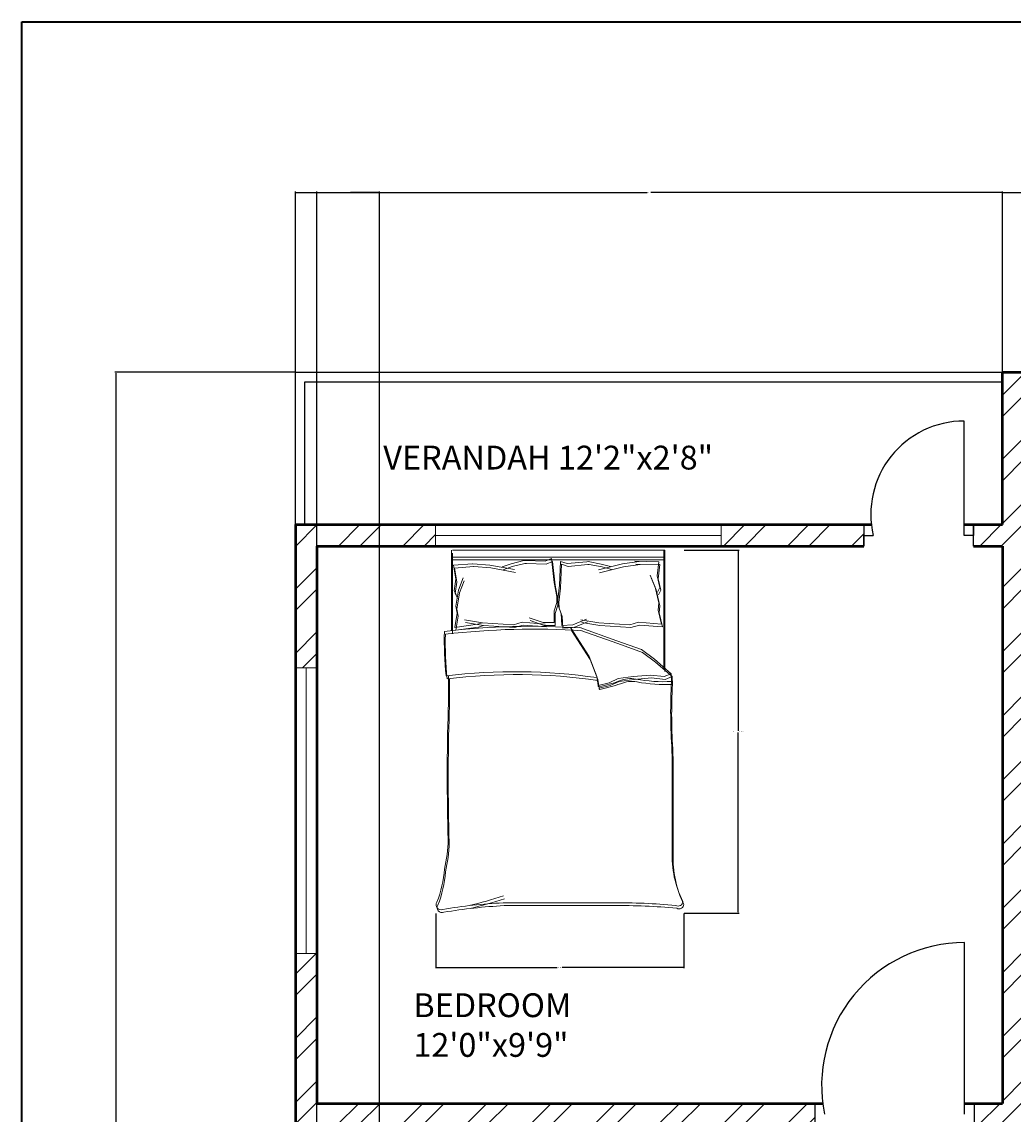
# Model space of a CAD drawing. Units: inches. Extents: x 2129 to 2642, y 1542 to 2414.
# Tile 6 of 9: x 2129 to 2338, y 2184 to 2414. Entities that reach past the tile are written whole.
import ezdxf

# ---------------------------------------------------------------- set-up
doc = ezdxf.new("R2010")
doc.units = ezdxf.units.IN
for name, color, linetype, lineweight in [('A-ANNO-DIMS', 2, 'Continuous', 18), ('A-ANNO-TTLB', 7, 'Continuous', 35), ('A-AREA-IDEN', 7, 'Continuous', 18), ('A-DOOR', 3, 'Continuous', 25), ('A-FLOR-RAIL', 80, 'Continuous', 25), ('A-FURN', 8, 'Continuous', 18), ('A-GLAZ', 4, 'Continuous', 18), ('A-WALL', 7, 'Continuous', 50), ('A-WALL-PATT', 252, 'Continuous', 13)]:
    doc.layers.add(name, color=color, linetype=linetype, lineweight=lineweight)
doc.styles.get("Standard").update_dxf_attribs({"font": 'arial.ttf'})
doc.dimstyles.get("Standard").update_dxf_attribs({"dimtxt": 0.18, "dimasz": 0.18, "dimexe": 0.18, "dimexo": 0.0625, "dimgap": 0.09, "dimtad": 0, "dimtih": 1, "dimtoh": 1, "dimdec": 4, "dimzin": 0, "dimdsep": 46, "dimtxsty": 'Standard', "dimcen": 0.09, "dimadec": 0, "dimazin": 0, "dimtfac": 1, "dimtdec": 4, "dimtofl": 0, "dimtmove": 0, "dimatfit": 3, "dimfxl": 1, "dimtolj": 1, "dimtzin": 0, "dimarcsym": 0})

# ---------------------------------------------------------------- blocks, each defined once
blk = doc.blocks.new('BED-DOUBLE')
for p, q in [((3.24, 59.14), (3.24, 76.05)), ((3.25, 59.14), (3.25, 76.05)), ((48.08, 76.05), (3.46, 76.05)), ((47.87, 76.05), (47.87, 51.2)), ((47.87, 76.05), (47.87, 51.2)), ((48.08, 76.05), (48.08, 75.45)), ((3.24, 74.61), (47.87, 74.61)), ((3.25, 74.61), (47.87, 74.61)), ((3.46, 58.54), (3.46, 75.45)), ((3.46, 58.54), (3.46, 75.45)), ((3.46, 74.02), (48.08, 74.02)), ((3.46, 74.02), (48.08, 74.02)), ((15.76, 73.22), (18.46, 73.9)), ((15.76, 73.22), (18.46, 73.9)), ((18.46, 73.9), (18.76, 73.9)), ((18.46, 73.9), (18.76, 73.9)), ((18.76, 73.9), (22.91, 73.76)), ((18.76, 73.9), (22.91, 73.76)), ((22.91, 73.76), (24.26, 74.3)), ((22.91, 73.76), (24.26, 74.3)), ((23.12, 73.16), (24.47, 73.7)), ((23.12, 73.16), (24.47, 73.7)), ((24.26, 74.3), (24.8, 69.31)), ((24.26, 74.3), (24.8, 69.31)), ((24.47, 73.7), (25.01, 68.71)), ((24.47, 73.7), (25.01, 68.71)), ((26.12, 73.72), (25.9, 68.7)), ((26.12, 73.72), (25.9, 68.7)), ((27.5, 73.27), (26.12, 73.72)), ((27.5, 73.27), (26.12, 73.72)), ((31.64, 73.66), (27.5, 73.27)), ((31.64, 73.66), (27.5, 73.27)), ((31.94, 73.68), (31.64, 73.66)), ((31.94, 73.68), (31.64, 73.66)), ((34.68, 73.17), (31.94, 73.68)), ((34.67, 73.17), (31.94, 73.68)), ((42.68, 73.67), (39.14, 73.18)), ((42.68, 73.67), (39.14, 73.18)), ((46.79, 73.66), (41.75, 73.75)), ((41.75, 73.75), (42.68, 73.67)), ((46.79, 73.66), (41.75, 73.75)), ((41.75, 73.75), (42.68, 73.67)), ((46.79, 73.66), (46.44, 70.66)), ((46.79, 73.66), (46.44, 70.66)), ((48.08, 75.45), (48.08, 50.6)), ((48.08, 75.45), (48.08, 50.6)), ((3.64, 72.93), (7.64, 73.24)), ((3.64, 72.93), (7.64, 73.24)), ((3.64, 72.95), (4.18, 69.98)), ((3.64, 72.95), (4.18, 69.98)), ((3.85, 72.33), (7.85, 72.64)), ((3.85, 72.33), (7.85, 72.64)), ((3.85, 72.35), (4.39, 69.38)), ((3.85, 72.35), (4.39, 69.38)), ((7.64, 73.24), (7.74, 73.22)), ((7.64, 73.24), (7.74, 73.22)), ((7.74, 73.22), (11.31, 72.95)), ((7.74, 73.22), (11.31, 72.95)), ((7.85, 72.64), (7.95, 72.62)), ((7.85, 72.64), (7.95, 72.62)), ((7.95, 72.62), (11.52, 72.35)), ((7.95, 72.62), (11.52, 72.35)), ((11.31, 72.95), (16.44, 72.01)), ((11.31, 72.95), (16.44, 72.01)), ((11.52, 72.35), (16.65, 71.41)), ((11.52, 72.35), (16.65, 71.41)), ((13.87, 72.55), (15.76, 73.22)), ((13.87, 72.55), (15.76, 73.22)), ((14.08, 71.95), (15.97, 72.62)), ((14.08, 71.95), (15.97, 72.62)), ((15.97, 72.62), (18.67, 73.3)), ((15.97, 72.62), (18.67, 73.3)), ((18.67, 73.3), (18.97, 73.3)), ((18.67, 73.3), (18.97, 73.3)), ((18.97, 73.3), (23.12, 73.16)), ((18.97, 73.3), (23.12, 73.16)), ((26.34, 73.12), (26.11, 68.1)), ((26.34, 73.12), (26.11, 68.1)), ((27.72, 72.67), (26.34, 73.12)), ((27.72, 72.67), (26.34, 73.12)), ((31.85, 73.06), (27.72, 72.67)), ((31.85, 73.06), (27.72, 72.67)), ((32.15, 73.08), (31.85, 73.06)), ((32.15, 73.08), (31.85, 73.06)), ((34.89, 72.58), (32.15, 73.08)), ((34.89, 72.58), (32.15, 73.08)), ((39.14, 73.18), (34.08, 71.92)), ((39.14, 73.18), (34.08, 71.92)), ((39.35, 72.58), (34.29, 71.32)), ((39.35, 72.58), (34.29, 71.32)), ((36.6, 72.62), (34.67, 73.17)), ((36.6, 72.62), (34.68, 73.17)), ((36.82, 72.02), (34.89, 72.58)), ((36.82, 72.02), (34.89, 72.58)), ((42.9, 73.08), (39.35, 72.58)), ((42.9, 73.08), (39.35, 72.58)), ((47.01, 73.06), (41.96, 73.15)), ((41.96, 73.15), (42.9, 73.08)), ((47.01, 73.06), (41.96, 73.15)), ((41.96, 73.15), (42.9, 73.08)), ((47.01, 73.06), (46.65, 70.06)), ((47.01, 73.06), (46.65, 70.06)), ((4.18, 69.98), (3.77, 67.55)), ((4.18, 69.98), (3.77, 67.55)), ((4.39, 69.38), (3.98, 66.95)), ((4.39, 69.38), (3.99, 66.95)), ((4.72, 67.69), (5.66, 70.25)), ((4.72, 67.69), (5.66, 70.25)), ((4.93, 67.09), (5.87, 69.65)), ((4.93, 67.09), (5.87, 69.65)), ((24.8, 69.31), (25.34, 66.34)), ((24.8, 69.31), (25.34, 66.34)), ((46.04, 68.34), (44.94, 70.84)), ((46.04, 68.34), (44.94, 70.84)), ((46.26, 67.74), (45.15, 70.24)), ((46.26, 67.74), (45.15, 70.24)), ((46.44, 70.66), (46.99, 68.26)), ((46.44, 70.66), (46.99, 68.26)), ((46.65, 70.06), (47.21, 67.66)), ((46.65, 70.06), (47.21, 67.66)), ((3.77, 67.55), (4.31, 66.61)), ((3.77, 67.55), (4.31, 66.61)), ((3.98, 66.95), (4.52, 66.01)), ((3.99, 66.95), (4.53, 66.01)), ((4.18, 64.31), (4.72, 67.69)), ((4.18, 64.31), (4.72, 67.69)), ((4.39, 63.71), (4.93, 67.09)), ((4.39, 63.71), (4.93, 67.09)), ((25.01, 68.71), (25.55, 65.74)), ((25.01, 68.71), (25.55, 65.74)), ((25.9, 68.7), (25.54, 65.7)), ((25.9, 68.7), (25.54, 65.7)), ((26.11, 68.1), (25.76, 65.11)), ((26.11, 68.1), (25.76, 65.11)), ((46.79, 65), (46.04, 68.34)), ((46.79, 65), (46.04, 68.34)), ((47.01, 64.41), (46.26, 67.74)), ((47.01, 64.41), (46.26, 67.74)), ((46.99, 68.26), (46.51, 67.28)), ((46.99, 68.26), (46.51, 67.28)), ((47.21, 67.66), (46.73, 66.69)), ((47.21, 67.66), (46.73, 66.69)), ((4.45, 62.82), (4.18, 64.31)), ((4.45, 62.82), (4.18, 64.31)), ((25.34, 65.12), (24.8, 63.36)), ((25.34, 65.12), (24.8, 63.36)), ((25.55, 64.52), (25.01, 62.77)), ((25.55, 64.52), (25.01, 62.77)), ((25.34, 66.34), (25.34, 65.12)), ((25.34, 66.34), (25.34, 65.12)), ((25.54, 65.7), (25.62, 64.49)), ((25.54, 65.7), (25.62, 64.49)), ((25.55, 65.74), (25.55, 64.52)), ((25.55, 65.74), (25.55, 64.52)), ((25.62, 64.49), (26.27, 62.77)), ((25.62, 64.49), (26.27, 62.77)), ((25.76, 65.11), (25.83, 63.89)), ((25.76, 65.11), (25.83, 63.89)), ((46.62, 63.5), (46.79, 65)), ((46.62, 63.5), (46.79, 65)), ((46.83, 62.91), (47.01, 64.41)), ((46.83, 62.91), (47.01, 64.41)), ((3.91, 59.85), (4.45, 62.82)), ((3.91, 59.85), (4.45, 62.82)), ((4.12, 59.26), (4.66, 62.23)), ((4.12, 59.26), (4.66, 62.23)), ((4.66, 62.23), (4.39, 63.71)), ((4.66, 62.23), (4.39, 63.71)), ((24.8, 63.36), (24.8, 60.86)), ((24.8, 63.36), (24.8, 60.86)), ((25.01, 62.77), (25.01, 60.26)), ((25.01, 62.77), (25.01, 60.26)), ((25.83, 63.89), (26.48, 62.18)), ((25.83, 63.89), (26.48, 62.18)), ((26.27, 62.77), (26.42, 60.27)), ((26.27, 62.77), (26.42, 60.27)), ((26.48, 62.18), (26.64, 59.68)), ((26.48, 62.18), (26.64, 59.68)), ((47.34, 60.57), (46.62, 63.5)), ((47.34, 60.57), (46.62, 63.5)), ((47.55, 59.98), (46.83, 62.91)), ((47.55, 59.98), (46.83, 62.91)), ((8.67, 60.53), (3.91, 59.85)), ((8.67, 60.53), (3.91, 59.85)), ((8.88, 59.93), (4.12, 59.26)), ((8.88, 59.93), (4.12, 59.26)), ((5.96, 61.45), (9.72, 60.83)), ((5.96, 61.45), (9.72, 60.83)), ((6.17, 60.86), (9.94, 60.23)), ((6.17, 60.86), (9.94, 60.23)), ((9.72, 60.83), (8.67, 60.53)), ((9.72, 60.83), (8.67, 60.53)), ((9.94, 60.23), (8.88, 59.93)), ((9.94, 60.23), (8.88, 59.93)), ((9.72, 60.83), (16.27, 60.43)), ((9.72, 60.83), (16.27, 60.43)), ((9.94, 60.23), (16.48, 59.83)), ((9.94, 60.23), (16.48, 59.83)), ((16.27, 60.43), (18.1, 60.95)), ((16.27, 60.43), (18.1, 60.95)), ((16.48, 59.83), (18.31, 60.35)), ((16.48, 59.83), (18.31, 60.35)), ((18.1, 60.95), (22.89, 60.57)), ((18.1, 60.95), (22.89, 60.57)), ((18.31, 60.35), (23.11, 59.98)), ((18.31, 60.35), (23.1, 59.98)), ((22.51, 60.86), (19.57, 61.88)), ((22.51, 60.86), (19.57, 61.88)), ((22.72, 60.26), (19.78, 61.28)), ((22.72, 60.26), (19.78, 61.28)), ((24.8, 60.86), (22.51, 60.86)), ((24.8, 60.86), (22.51, 60.86)), ((25.01, 60.26), (22.72, 60.26)), ((25.01, 60.26), (22.72, 60.26)), ((26.42, 60.27), (28.71, 60.42)), ((26.42, 60.27), (28.71, 60.42)), ((26.64, 59.68), (28.93, 59.82)), ((26.64, 59.68), (28.93, 59.82)), ((28.25, 59.82), (32.17, 53.75)), ((28.25, 59.82), (32.17, 53.75)), ((28.71, 60.42), (31.58, 61.62)), ((28.71, 60.42), (31.58, 61.62)), ((28.93, 59.82), (31.79, 61.02)), ((28.93, 59.82), (31.79, 61.02)), ((37.95, 57.08), (30.17, 59.82)), ((37.95, 57.08), (30.17, 59.82)), ((30.41, 61.45), (34.17, 60.83)), ((30.41, 61.45), (34.17, 60.83)), ((30.62, 60.86), (34.39, 60.23)), ((30.62, 60.86), (34.38, 60.23)), ((34.17, 60.83), (40.72, 60.43)), ((34.17, 60.83), (40.72, 60.43)), ((34.38, 60.23), (40.93, 59.83)), ((34.39, 60.23), (40.93, 59.83)), ((40.72, 60.43), (42.55, 60.95)), ((40.72, 60.43), (42.55, 60.95)), ((40.93, 59.83), (42.76, 60.35)), ((40.93, 59.83), (42.76, 60.35)), ((42.55, 60.95), (47.34, 60.57)), ((42.55, 60.95), (47.34, 60.57)), ((42.76, 60.35), (47.55, 59.98)), ((42.76, 60.35), (47.55, 59.98)), ((28.47, 59.22), (32.38, 53.16)), ((28.47, 59.22), (32.38, 53.16)), ((38.16, 56.48), (30.38, 59.22)), ((38.16, 56.48), (30.38, 59.22)), ((43.16, 55.2), (37.95, 57.08)), ((43.16, 55.2), (37.95, 57.08)), ((43.37, 54.6), (38.16, 56.48)), ((43.37, 54.6), (38.16, 56.48)), ((45.91, 53.17), (43.16, 55.2)), ((45.91, 53.17), (43.16, 55.2)), ((32.17, 53.75), (33.76, 49.56)), ((32.17, 53.75), (33.76, 49.56)), ((32.38, 53.16), (33.97, 48.96)), ((32.38, 53.16), (33.97, 48.96)), ((46.12, 52.58), (43.37, 54.6)), ((46.12, 52.58), (43.37, 54.6)), ((49.37, 50.14), (45.91, 53.17)), ((49.36, 50.14), (45.91, 53.17)), ((49.58, 49.54), (46.12, 52.58)), ((49.58, 49.54), (46.12, 52.58)), ((33.76, 49.56), (34.05, 47.68)), ((33.76, 49.56), (34.05, 47.68)), ((33.97, 48.96), (34.26, 47.09)), ((33.97, 48.96), (34.26, 47.09)), ((34.05, 47.68), (36.36, 48.26)), ((34.05, 47.68), (36.36, 48.26)), ((36.36, 48.26), (38.24, 49.13)), ((36.36, 48.26), (38.24, 49.13)), ((36.57, 47.66), (38.45, 48.53)), ((36.57, 47.66), (38.45, 48.53)), ((38.24, 49.13), (41.42, 49.56)), ((38.24, 49.13), (41.42, 49.56)), ((38.45, 48.53), (41.64, 48.96)), ((38.45, 48.53), (41.64, 48.96)), ((41.42, 49.56), (45.04, 49.85)), ((41.42, 49.56), (45.04, 49.85)), ((41.64, 48.96), (45.25, 49.25)), ((41.64, 48.96), (45.25, 49.25)), ((45.04, 49.85), (47.93, 49.56)), ((45.04, 49.85), (47.93, 49.56)), ((45.25, 49.25), (48.14, 48.96)), ((45.25, 49.25), (48.14, 48.96)), ((47.93, 49.56), (49.37, 50.14)), ((47.93, 49.56), (49.36, 50.14)), ((48.14, 48.96), (49.58, 49.54)), ((48.14, 48.96), (49.58, 49.54)), ((49.44, 48.51), (49.36, 50.14, 3.61)), ((49.44, 48.51), (49.37, 50.14, 3.61)), ((49.65, 47.91), (49.58, 49.54, 3.61)), ((49.65, 47.91), (49.58, 49.54, 3.61)), ((34.26, 47.09), (36.57, 47.66)), ((34.26, 47.09), (36.57, 47.66)), ((14.07, 2.05), (37.05, 2.05)), ((14.07, 2.05), (37.05, 2.05)), ((14.28, 1.46), (37.26, 1.46)), ((14.28, 1.46), (37.26, 1.46))]:
    blk.add_line(p, q)
for centre, radius, start, end in [((19.94, -93.94), 154.04, 86.0865, 96.7821), ((19.94, -93.94), 154.04, 86.0865, 96.7821), ((79.52, 57.28), 77.79, 178.7218, 185.604), ((79.52, 57.28), 77.79, 178.7218, 185.604), ((79.73, 56.69), 77.79, 178.7218, 185.604), ((79.73, 56.69), 77.79, 178.7218, 185.604), ((20.16, -94.54), 154.04, 86.0865, 96.7821), ((20.16, -94.54), 154.04, 86.0865, 96.7821), ((16.58, -69.91), 120.47, 81.7845, 96.9006), ((16.58, -69.91), 120.47, 81.7845, 96.9006), ((16.79, -70.51), 120.47, 81.7845, 96.9006), ((16.79, -70.51), 120.47, 81.7845, 96.9006), ((-156.22, 46.94), 158.84, 358.4762, 1.0082), ((-156.22, 46.94), 158.84, 358.4762, 1.0082), ((-156.01, 46.34), 158.84, 358.4762, 1.0082), ((-156.01, 46.34), 158.84, 358.4762, 1.0082), ((29.09, 74.66), 27.69, 280.6617, 289.8806), ((29.09, 74.66), 27.69, 280.6617, 289.8806), ((40.85, 43.3), 5.81, 78.6608, 113.7384), ((40.85, 43.3), 5.81, 78.6608, 113.7384), ((41.06, 42.71), 5.81, 78.6608, 113.7384), ((41.06, 42.71), 5.81, 78.6608, 113.7384), ((47.93, 82.26), 33.79, 259.8763, 272.5657), ((47.93, 82.26), 33.79, 259.8763, 272.5657), ((48.14, 81.67), 33.79, 259.8763, 272.5657), ((48.14, 81.67), 33.79, 259.8763, 272.5657), ((170.19, 42.14), 120.92, 176.9791, 183.8365), ((170.19, 42.14), 120.92, 176.9791, 183.8365), ((34.21, 47.62), 0.172, 160.2464, 271.1377), ((34.21, 47.62), 0.172, 160.2464, 271.1377), ((34.42, 47.03), 0.172, 160.2464, 271.1377), ((34.42, 47.03), 0.172, 160.2464, 271.1377), ((29.3, 74.07), 27.69, 280.6617, 289.8806), ((29.3, 74.07), 27.69, 280.6617, 289.8806), ((170.4, 41.54), 120.92, 176.9791, 183.8365), ((170.4, 41.54), 120.92, 176.9791, 183.8365), ((452.7, 28.79), 450.36, 178.2277, 181.7185), ((452.7, 28.79), 450.36, 178.2277, 181.7185), ((452.91, 28.19), 450.36, 178.2277, 181.7185), ((452.91, 28.19), 450.36, 178.2277, 181.7185), ((-4210.02, 12.72), 4259.62, 0.00217, 0.28689), ((-4210.02, 12.72), 4259.62, 0.00217, 0.28689), ((-4209.81, 12.12), 4259.62, 0.00217, 0.28689), ((-4209.81, 12.12), 4259.62, 0.00217, 0.28689), ((-25.12, 15.81), 27.67, 346.0648, 358.9113), ((-25.12, 15.81), 27.67, 346.0648, 358.9113), ((-24.9, 15.21), 27.67, 346.0648, 358.9113), ((-24.9, 15.21), 27.67, 346.0648, 358.9113), ((71.11, 11.93), 21.54, 177.4714, 206.4681), ((71.11, 11.93), 21.54, 177.4714, 206.4681), ((71.33, 11.33), 21.54, 177.4714, 206.4681), ((71.32, 11.33), 21.54, 177.4714, 206.4681), ((-20.22, 10.43), 22, 337.9751, 356.652), ((-20.22, 10.43), 22, 337.9751, 356.652), ((-20.01, 9.83), 22, 337.9751, 356.652), ((-20.01, 9.83), 22, 337.9751, 356.652), ((-16.08, 98.19), 99.41, 283.3832, 287.7053), ((-16.08, 98.19), 99.41, 283.3832, 287.7053), ((-15.87, 97.59), 99.41, 283.3832, 287.7053), ((-15.87, 97.59), 99.41, 283.3832, 287.7053), ((50.81, 2.4), 1.03, 242.6588, 356.02), ((50.81, 2.4), 1.03, 242.6588, 356.02), ((1.02, 1.61), 1.02, 146.1736, 293.4781), ((1.02, 1.61), 1.02, 146.1736, 293.4781), ((1.23, 1.01), 1.02, 146.1736, 293.4781), ((1.23, 1.01), 1.02, 146.1736, 293.4781), ((20.01, -111.48), 113.69, 92.9958, 99.4091), ((20.01, -111.48), 113.69, 92.9958, 99.4091), ((20.22, -112.08), 113.69, 92.9958, 99.4091), ((20.22, -112.08), 113.69, 92.9958, 99.4091), ((38.43, -122.17), 124.23, 84.4998, 90.6351), ((38.43, -122.17), 124.23, 84.4998, 90.6351), ((38.64, -122.76), 124.23, 84.4998, 90.6351), ((38.64, -122.76), 124.23, 84.4998, 90.6351), ((51.02, 1.81), 1.03, 242.6588, 356.02), ((51.02, 1.81), 1.03, 242.6588, 356.02)]:
    blk.add_arc(centre, radius, start, end)
blk = doc.blocks.new('WIN-60-A')
for p, q in [((0, 4.5), (0, 0)), ((60, 2.25), (60, 4.5)), ((60, 4.5), (60, 0)), ((0, 0), (0, 2.25)), ((0, 2.25), (60, 2.25))]:
    blk.add_line(p, q)
blk = doc.blocks.new('*D12')
at = {"layer": 'A-ANNO-DIMS', "color": 0, "lineweight": -2, "transparency": 16777216}
for p, q in [((2268.55, 2302.83), (2280.09, 2302.83)), ((2279.91, 2302.65), (2279.91, 2264.94)), ((2279.91, 2226.87), (2279.91, 2264.58)), ((2268.55, 2226.69), (2280.09, 2226.69))]:
    blk.add_line(p, q, dxfattribs=at)
at = {"layer": 'A-ANNO-DIMS', "color": 0, "transparency": 16777216}
for points in [[(2279.88, 2302.65), (2279.94, 2302.65), (2279.91, 2302.83)], [(2279.88, 2226.87), (2279.94, 2226.87), (2279.91, 2226.69)]]:
    blk.add_solid(points, dxfattribs=at)
at = {"layer": 'Defpoints', "color": 0, "transparency": 16777216}
for p in [(2268.49, 2302.83), (2279.91, 2302.83), (2268.49, 2226.69)]:
    blk.add_point(p, dxfattribs=at)
at = {"layer": 'A-ANNO-DIMS', "color": 0, "transparency": 16777216, "insert": (2279.91, 2264.76), "char_height": 0.18, "attachment_point": 5}
blk.add_mtext('\\A1;DOUBLE BED 76 TYP.', dxfattribs=at)
blk = doc.blocks.new('*D13')
at = {"layer": 'A-ANNO-DIMS', "color": 0, "lineweight": -2, "transparency": 16777216}
for p, q in [((2216.36, 2226.62), (2216.36, 2215.09)), ((2268.49, 2226.62), (2268.49, 2215.09)), ((2216.54, 2215.27), (2241.9, 2215.27)), ((2268.31, 2215.27), (2242.96, 2215.27))]:
    blk.add_line(p, q, dxfattribs=at)
at = {"layer": 'A-ANNO-DIMS', "color": 0, "transparency": 16777216}
for points in [[(2216.54, 2215.3), (2216.54, 2215.24), (2216.36, 2215.27)], [(2268.31, 2215.3), (2268.31, 2215.24), (2268.49, 2215.27)]]:
    blk.add_solid(points, dxfattribs=at)
at = {"layer": 'Defpoints', "color": 0, "transparency": 16777216}
for p in [(2216.36, 2226.69), (2268.49, 2226.69), (2268.49, 2215.27)]:
    blk.add_point(p, dxfattribs=at)
at = {"layer": 'A-ANNO-DIMS', "color": 0, "transparency": 16777216, "insert": (2242.43, 2215.27), "char_height": 0.18, "attachment_point": 5}
blk.add_mtext('\\A1;52 TYP.', dxfattribs=at)
blk = doc.blocks.new('*D35')
at = {"layer": 'A-ANNO-DIMS', "color": 0, "lineweight": -2, "transparency": 16777216}
for p, q in [((2186.84, 2340.22), (2148.97, 2340.22)), ((2149.15, 2340.04), (2149.15, 2003.15)), ((2149.15, 1665.9), (2149.15, 2002.79)), ((2186.84, 1665.72), (2148.97, 1665.72))]:
    blk.add_line(p, q, dxfattribs=at)
at = {"layer": 'A-ANNO-DIMS', "color": 0, "transparency": 16777216}
for points in [[(2149.12, 2340.04), (2149.18, 2340.04), (2149.15, 2340.22)], [(2149.12, 1665.9), (2149.18, 1665.9), (2149.15, 1665.72)]]:
    blk.add_solid(points, dxfattribs=at)
at = {"layer": 'Defpoints', "color": 0, "transparency": 16777216}
for p in [(2149.15, 2340.22), (2186.9, 2340.22), (2186.9, 1665.72)]:
    blk.add_point(p, dxfattribs=at)
at = {"layer": 'A-ANNO-DIMS', "color": 0, "transparency": 16777216, "insert": (2149.15, 2002.97), "char_height": 0.18, "attachment_point": 5}
blk.add_mtext('\\A1;674.5', dxfattribs=at)
blk = doc.blocks.new('*D36')
at = {"layer": 'A-ANNO-DIMS', "color": 0, "lineweight": -2, "transparency": 16777216}
for p, q in [((2186.9, 2340.28), (2186.9, 2378.15)), ((2187.08, 2377.97), (2260.77, 2377.97)), ((2335.22, 2377.97), (2261.54, 2377.97)), ((2335.4, 2340.28), (2335.4, 2378.15))]:
    blk.add_line(p, q, dxfattribs=at)
at = {"layer": 'A-ANNO-DIMS', "color": 0, "transparency": 16777216}
for points in [[(2187.08, 2378), (2187.08, 2377.94), (2186.9, 2377.97)], [(2335.22, 2378), (2335.22, 2377.94), (2335.4, 2377.97)]]:
    blk.add_solid(points, dxfattribs=at)
at = {"layer": 'Defpoints', "color": 0, "transparency": 16777216}
for p in [(2335.4, 2377.97), (2186.9, 2340.22), (2335.4, 2340.22)]:
    blk.add_point(p, dxfattribs=at)
at = {"layer": 'A-ANNO-DIMS', "color": 0, "transparency": 16777216, "insert": (2261.15, 2377.97), "char_height": 0.18, "attachment_point": 5}
blk.add_mtext('\\A1;148.5', dxfattribs=at)
blk = doc.blocks.new('*D37')
at = {"layer": 'A-ANNO-DIMS', "color": 0, "lineweight": -2, "transparency": 16777216}
for p, q in [((2335.4, 2340.28), (2335.4, 2378.15)), ((2335.58, 2377.97), (2387.62, 2377.97)), ((2440.22, 2377.97), (2388.19, 2377.97)), ((2440.4, 2340.28), (2440.4, 2378.15))]:
    blk.add_line(p, q, dxfattribs=at)
at = {"layer": 'A-ANNO-DIMS', "color": 0, "transparency": 16777216}
for points in [[(2335.58, 2378), (2335.58, 2377.94), (2335.4, 2377.97)], [(2440.22, 2378), (2440.22, 2377.94), (2440.4, 2377.97)]]:
    blk.add_solid(points, dxfattribs=at)
at = {"layer": 'Defpoints', "color": 0, "transparency": 16777216}
for p in [(2440.4, 2377.97), (2335.4, 2340.22), (2440.4, 2340.22)]:
    blk.add_point(p, dxfattribs=at)
at = {"layer": 'A-ANNO-DIMS', "color": 0, "transparency": 16777216, "insert": (2387.9, 2377.97), "char_height": 0.18, "attachment_point": 5}
blk.add_mtext('\\A1;105', dxfattribs=at)
blk = doc.blocks.new('*D48')
at = {"layer": 'A-ANNO-DIMS', "color": 0, "lineweight": -2, "transparency": 16777216}
for p, q in [((2191.4, 2007.28), (2191.4, 2378.15)), ((2191.58, 2377.97), (2197.54, 2377.97)), ((2204.41, 2377.97), (2198.45, 2377.97)), ((2204.59, 2007.28), (2204.59, 2378.15))]:
    blk.add_line(p, q, dxfattribs=at)
at = {"layer": 'A-ANNO-DIMS', "color": 0, "transparency": 16777216}
for points in [[(2191.58, 2378), (2191.58, 2377.94), (2191.4, 2377.97)], [(2204.41, 2378), (2204.41, 2377.94), (2204.59, 2377.97)]]:
    blk.add_solid(points, dxfattribs=at)
at = {"layer": 'Defpoints', "color": 0, "transparency": 16777216}
for p in [(2204.59, 2377.97), (2191.4, 2007.22), (2204.59, 2007.22)]:
    blk.add_point(p, dxfattribs=at)
at = {"layer": 'A-ANNO-DIMS', "color": 0, "transparency": 16777216, "insert": (2198, 2377.97), "char_height": 0.18, "attachment_point": 5}
blk.add_mtext('\\A1;13.186', dxfattribs=at)

msp = doc.modelspace()

# ---------------------------------------------------------------- hatches: boundary and pattern name
at = {"layer": 'A-WALL-PATT'}
h = msp.add_hatch(dxfattribs=at)
h.set_pattern_fill('ANSI32', color=256)
h.paths.add_polyline_path([(2306.2606, 2305.9717), (2306.2606, 2308.2217), (2276.3515, 2308.2217), (2276.3515, 2303.7217), (2306.2606, 2303.7217)])
h.paths.add_polyline_path([(2216.3515, 2305.9717), (2216.3515, 2308.2217), (2186.9043, 2308.2217), (2186.9043, 2278.1696), (2191.4043, 2278.1696), (2191.4043, 2303.7217), (2216.3515, 2303.7217)])
h.paths.add_polyline_path([(2339.9043, 2335.7217), (2362.1938, 2335.7217), (2362.1938, 2340.2217), (2335.4043, 2340.2217), (2335.4043, 2308.2217), (2329.3487, 2308.2217), (2329.3487, 2305.9717), (2329.3487, 2303.7217), (2335.4043, 2303.7217), (2335.4043, 2186.7217), (2329.4345, 2186.7217), (2329.4345, 2182.2217), (2335.4043, 2182.2217), (2335.4043, 2174.7178), (2339.9043, 2174.7178), (2339.9043, 2182.2217), (2339.9043, 2303.7217)])
h.paths.add_polyline_path([(2440.4043, 2340.2217), (2411.654, 2340.2217), (2411.654, 2335.7217), (2435.9043, 2335.7217), (2435.9043, 2303.7217), (2435.9043, 2182.2217), (2435.9043, 2174.1935), (2438.1543, 2174.1935), (2440.4043, 2174.1935), (2440.4043, 2182.2217), (2444.653, 2182.2217), (2444.653, 2184.4717), (2444.653, 2186.7217), (2440.4043, 2186.7217), (2440.4043, 2303.7217), (2445.8547, 2303.7217), (2445.8547, 2308.2217), (2440.4043, 2308.2217)])
h.paths.add_polyline_path([(2498.2381, 2308.2217), (2470.3901, 2308.2217), (2470.3901, 2303.7217), (2498.2381, 2303.7217), (2498.2381, 2305.9717)])
h.paths.add_polyline_path([(2588.9043, 2308.2217), (2586.9043, 2308.2217), (2558.2381, 2308.2217), (2558.2381, 2303.7217), (2584.4043, 2303.7217), (2584.4043, 2279.1087), (2588.9043, 2279.1087)])
h.paths.add_polyline_path([(2588.9043, 2219.1087), (2584.4043, 2219.1087), (2584.4043, 2186.7217), (2478.0667, 2186.7217), (2478.0667, 2182.2217), (2584.4043, 2182.2217), (2584.4043, 2157.7883), (2588.9043, 2157.7883)])
h.paths.add_polyline_path([(2588.9043, 2097.7883), (2584.6063, 2097.7883), (2584.6063, 2075.5462, -0.09241561), (2584.4043, 2074.4627), (2584.4043, 2064.2217), (2495.9043, 2064.2217), (2495.9043, 2040.4611), (2500.4043, 2040.4611), (2500.4043, 2059.7217), (2584.4043, 2059.7217), (2584.4043, 2052.2164), (2588.9043, 2052.2164)])
h.paths.add_polyline_path([(2588.9043, 2028.2164), (2584.4043, 2028.2164), (2584.4043, 2011.7217), (2500.4043, 2011.7217), (2500.4043, 2015.243), (2498.1543, 2015.243), (2495.9043, 2015.243), (2495.9043, 2007.2217), (2495.9043, 2003.7597), (2500.4043, 2003.7597), (2500.4043, 2007.2217), (2584.4043, 2007.2217), (2584.4043, 1992.1997), (2588.9043, 1992.1997)])
h.paths.add_polyline_path([(2588.9043, 1956.1997), (2584.4043, 1956.1997), (2584.4043, 1941.2217), (2500.4043, 1941.2217), (2500.4043, 1985.1493), (2498.1543, 1985.1493), (2495.9043, 1985.1493), (2495.9043, 1941.2217), (2435.9043, 1941.2217), (2435.9043, 1930.3963), (2440.4043, 1930.3963), (2440.4043, 1936.7217), (2584.4043, 1936.7217), (2584.4043, 1909.8406), (2588.9043, 1909.8406)])
h.paths.add_polyline_path([(2588.9043, 1849.8406), (2584.4043, 1849.8406), (2584.4043, 1801.3526), (2588.9043, 1801.3526)])
h.paths.add_polyline_path([(2584.4043, 1828.7217), (2495.9043, 1828.7217), (2440.4043, 1828.7217), (2440.4043, 1905.2159), (2438.1543, 1905.2159), (2435.9043, 1905.2159), (2435.9043, 1828.7217), (2428.9101, 1828.7217), (2428.9101, 1824.2217), (2584.4043, 1824.2217)])
h.paths.add_polyline_path([(2588.9043, 1741.3526), (2584.4043, 1741.3526), (2584.4043, 1704.2217), (2468.3173, 1704.2217), (2468.3173, 1701.9717), (2468.3173, 1699.7217), (2588.9043, 1699.7217)])
h.paths.add_polyline_path([(2442.4043, 1761.7217), (2435.0216, 1761.7217), (2435.0216, 1757.2217), (2437.9043, 1757.2217), (2437.9043, 1665.7217), (2442.4043, 1665.7217), (2442.4043, 1667.7217), (2442.4043, 1699.7217), (2446.6907, 1699.7217), (2446.6907, 1701.9717), (2446.6907, 1704.2217), (2442.4043, 1704.2217)])
h.paths.add_polyline_path([(2390.4043, 1757.2217), (2410.8996, 1757.2217), (2410.8996, 1761.7217), (2360.1741, 1761.7217), (2360.1741, 1759.4717), (2360.1741, 1757.2217), (2385.9043, 1757.2217), (2385.9043, 1674.8326), (2390.4043, 1674.8326)])
h.paths.add_polyline_path([(2337.9043, 1757.2217), (2340.3592, 1757.2217), (2340.3592, 1759.4717), (2340.3592, 1761.7217), (2333.4043, 1761.7217), (2333.4043, 1704.2217), (2327.381, 1704.2217), (2327.381, 1701.9717), (2327.381, 1699.7217), (2333.4043, 1699.7217), (2333.4043, 1665.7217), (2337.9043, 1665.7217)])
h.paths.add_polyline_path([(2191.4043, 1743.4804), (2186.9043, 1743.4804), (2186.9043, 1699.7217), (2188.9043, 1699.7217), (2191.4043, 1699.7217), (2306.5617, 1699.7217), (2306.5617, 1704.2217), (2191.4043, 1704.2217)])
h.paths.add_polyline_path([(2191.4043, 1859.8992), (2186.9043, 1859.8992), (2186.9043, 1803.4804), (2189.1543, 1803.4804), (2191.4043, 1803.4804)])
h.paths.add_polyline_path([(2352.5445, 1828.7217), (2191.4043, 1828.7217), (2191.4043, 1824.2217), (2333.4043, 1824.2217), (2352.5445, 1824.2217), (2352.5445, 1826.4717)])
h.paths.add_polyline_path([(2390.4043, 2085.328), (2385.9043, 2085.328), (2385.9043, 1828.7217), (2381.9668, 1828.7217), (2381.9668, 1826.4717), (2381.9668, 1824.2217), (2385.9043, 1824.2217), (2385.9043, 1761.7217), (2390.4043, 1761.7217), (2390.4043, 1824.2217), (2394.1868, 1824.2217), (2394.1868, 1827.6339), (2394.1868, 1828.7217), (2390.4043, 1828.7217)])
h.paths.add_polyline_path([(2339.9043, 1941.2217), (2335.4043, 1941.2217), (2279.9043, 1941.2217), (2279.9043, 1981.3432), (2277.6543, 1981.3432), (2275.4043, 1981.3432), (2275.4043, 1941.2217), (2191.4043, 1941.2217), (2191.4043, 1958.1079), (2186.9043, 1958.1079), (2186.9043, 1919.8992), (2189.1543, 1919.8992), (2191.4043, 1919.8992), (2191.4043, 1936.7217), (2279.9043, 1936.7217), (2335.4043, 1936.7217), (2335.4043, 1931.1382), (2339.9043, 1931.1382)])
h.paths.add_polyline_path([(2339.9043, 1902.7544), (2337.6543, 1902.7544), (2335.4043, 1902.7544), (2335.4043, 1828.7217), (2339.9043, 1828.7217)])
h.paths.add_polyline_path([(2279.9043, 2015.263), (2277.6543, 2015.263), (2275.4043, 2015.263), (2275.4043, 2011.7217), (2191.4043, 2011.7217), (2191.4043, 2026.6781), (2186.9043, 2026.6781), (2186.9043, 1994.1079), (2189.1543, 1994.1079), (2191.4043, 1994.1079), (2191.4043, 2007.2217), (2275.4043, 2007.2217), (2275.4043, 2003.2288), (2279.9043, 2003.2288), (2279.9043, 2007.2217)])
h.paths.add_polyline_path([(2296.0216, 2186.7217), (2191.4043, 2186.7217), (2191.4043, 2218.1696), (2186.9043, 2218.1696), (2186.9043, 2158.4509), (2191.4043, 2158.4509), (2191.4043, 2182.2217), (2296.0216, 2182.2217), (2296.0216, 2184.4717)])
h.paths.add_polyline_path([(2191.4043, 2098.4509), (2189.1543, 2098.4509), (2186.9043, 2098.4509), (2186.9043, 2050.6781), (2189.0487, 2050.6781), (2191.4043, 2050.6781), (2191.4043, 2059.7217), (2275.4043, 2059.7217), (2275.4043, 2038.4133), (2279.9043, 2038.4133), (2279.9043, 2064.2217), (2191.4043, 2064.2217)])
h.paths.add_polyline_path([(2268.3923, 1605.9386), (2516.3159, 1605.9386), (2516.3159, 1643.0314), (2268.3923, 1643.0314)], flags=9)
h.paths.add_polyline_path([(2399.6079, 1710.4489), (2428.8405, 1710.4489), (2428.8405, 1729.1062), (2399.6079, 1729.1062)], flags=9)
h.paths.add_polyline_path([(2342.1483, 1708.9956), (2371.3809, 1708.9956), (2371.3809, 1727.653), (2342.1483, 1727.653)], flags=9)
h.paths.add_polyline_path([(2200.7404, 1677.2519), (2282.3059, 1677.2519), (2282.3059, 1687.5555), (2200.7404, 1687.5555)], flags=9)
h.paths.add_polyline_path([(2209.8153, 1704.7448), (2250.627, 1704.7448), (2250.627, 1723.4021), (2209.8153, 1723.4021)], flags=25)
h.paths.add_polyline_path([(2213.9996, 1911.284), (2252.84, 1911.284), (2252.84, 1929.9413), (2213.9996, 1929.9413)], flags=9)
h.paths.add_polyline_path([(2210.8865, 1962.0987), (2244.0447, 1962.0987), (2244.0447, 1980.7561), (2210.8865, 1980.7561)], flags=25)
h.paths.add_polyline_path([(2219.0745, 2037.6131), (2248.2321, 2037.6131), (2248.2321, 2056.2705), (2219.0745, 2056.2705)], flags=9)
h.paths.add_polyline_path([(2379.9702, 2099.0686), (2409.3767, 2099.0686), (2409.3767, 2117.7259), (2379.9702, 2117.7259)], flags=9)
h.paths.add_polyline_path([(2375.9312, 2160.3752), (2405.3173, 2160.3752), (2405.3173, 2179.0325), (2375.9312, 2179.0325)], flags=9)
h.paths.add_polyline_path([(2269.5058, 2112.1824), (2310.3175, 2112.1824), (2310.3175, 2130.8397), (2269.5058, 2130.8397)], flags=9)
h.paths.add_polyline_path([(2209.6567, 2193.667), (2248.4971, 2193.667), (2248.4971, 2212.3243), (2209.6567, 2212.3243)], flags=25)
h.paths.add_polyline_path([(2491.6289, 1675.447), (2573.1944, 1675.447), (2573.1944, 1685.7506), (2491.6289, 1685.7506)], flags=9)
h.paths.add_polyline_path([(2492.0585, 1710.4489), (2530.8989, 1710.4489), (2530.8989, 1729.1062), (2492.0585, 1729.1062)], flags=25)
h.paths.add_polyline_path([(2495.6634, 1908.8646), (2534.5038, 1908.8646), (2534.5038, 1927.522), (2495.6634, 1927.522)], flags=9)
h.paths.add_polyline_path([(2516.7779, 1955.9942), (2549.9362, 1955.9942), (2549.9362, 1974.6516), (2516.7779, 1974.6516)], flags=25)
h.paths.add_polyline_path([(2509.7444, 2034.6896), (2538.902, 2034.6896), (2538.902, 2053.347), (2509.7444, 2053.347)], flags=9)
h.paths.add_polyline_path([(2467.8454, 2111.9593), (2508.6571, 2111.9593), (2508.6571, 2130.6167), (2467.8454, 2130.6167)], flags=9)
h.paths.add_polyline_path([(2528.5267, 2189.1742), (2567.3671, 2189.1742), (2567.3671, 2207.8316), (2528.5267, 2207.8316)], flags=25)
h.paths.add_polyline_path([(2483.7603, 2319.9841), (2557.5563, 2319.9841), (2557.5563, 2330.2877), (2483.7603, 2330.2877)], flags=9)
h.paths.add_polyline_path([(2204.078, 2317.0445), (2277.874, 2317.0445), (2277.874, 2327.3481), (2204.078, 2327.3481)], flags=9)

# ---------------------------------------------------------------- linework, layer by layer
at = {"layer": 'A-ANNO-TTLB'}
msp.add_lwpolyline([(2129.4387, 2413.7704), (2642.2731, 2413.7704), (2642.2731, 1542.3836), (2129.4387, 1542.3836)], close=True, dxfattribs=at)
at = {"layer": 'A-DOOR'}
for p, q in [((2327.3487, 2305.9717), (2327.3487, 2329.9717)), ((2306.2606, 2308.2217), (2306.2606, 2303.7217)), ((2329.3487, 2303.7217), (2329.3487, 2308.2217)), ((2329.3487, 2308.2217), (2329.3487, 2305.9717)), ((2306.2606, 2303.7217), (2306.2606, 2305.9717)), ((2306.2606, 2305.9717), (2308.2606, 2305.9717)), ((2329.3487, 2305.9717), (2327.3487, 2305.9717)), ((2327.4345, 2184.4717), (2327.4345, 2220.4717)), ((2296.0216, 2186.7217), (2296.0216, 2182.2217)), ((2329.4345, 2186.7217), (2329.4345, 2182.2217))]:
    msp.add_line(p, q, dxfattribs=at)
for centre, radius, end in [((2327.3487, 2310.3809), 19.5908, 193.006665), ((2327.4345, 2190.4562), 30.0155, 191.500693)]:
    msp.add_arc(centre, radius, 90, end, dxfattribs=at)
at = {"layer": 'A-FLOR-RAIL'}
for p, q in [((2186.9043, 2308.2217), (2186.9043, 2340.2217)), ((2186.9043, 2340.2217), (2335.4043, 2340.2217)), ((2188.9043, 2308.2217), (2188.9043, 2338.2217)), ((2188.9043, 2338.2217), (2335.4043, 2338.2217))]:
    msp.add_line(p, q, dxfattribs=at)
at = {"layer": 'A-WALL'}
for p, q in [((2335.4043, 2308.2217), (2335.4043, 2340.2217)), ((2335.4043, 2340.2217), (2362.1938, 2340.2217)), ((2186.9043, 2308.2217), (2307.8773, 2308.2217)), ((2186.9043, 2308.2217), (2307.8773, 2308.2217)), ((2186.9043, 2308.2217), (2186.9043, 1699.7217)), ((2186.9043, 2308.2217), (2186.9043, 2308.2217)), ((2186.9043, 2308.2217), (2188.9043, 2308.2217)), ((2327.3487, 2308.2217), (2335.4043, 2308.2217)), ((2327.3487, 2308.2217), (2335.4043, 2308.2217)), ((2191.4043, 2303.7217), (2306.2606, 2303.7217)), ((2191.4043, 2303.7217), (2191.4043, 2186.7217)), ((2329.3487, 2303.7217), (2335.4043, 2303.7217)), ((2335.4043, 2303.7217), (2335.4043, 2186.7217)), ((2191.4043, 2186.7217), (2297.6522, 2186.7217)), ((2327.4345, 2186.7217), (2335.4043, 2186.7217))]:
    msp.add_line(p, q, dxfattribs=at)

# ---------------------------------------------------------------- block references
at = {"layer": 'A-FURN'}
msp.add_blockref('BED-DOUBLE', (2216.445, 2226.786), dxfattribs=at)
at = {"layer": 'A-GLAZ'}
msp.add_blockref('WIN-60-A', (2216.352, 2303.722), dxfattribs=at)
at = {"layer": 'A-GLAZ', "rotation": 270.0000000000008}
msp.add_blockref('WIN-60-A', (2186.9047, 2278.1691), dxfattribs=at)

# ---------------------------------------------------------------- texts
at = {"layer": 'A-AREA-IDEN', "char_height": 5, "attachment_point": 1}
for s, width, insert in [('VERANDAH 12\'2"x2\'8"', 95.410861, (2205.3587, 2324.7952)), ('BEDROOM\\P12\'0"x9\'9"', 211.098193, (2211.6673, 2209.8397))]:
    msp.add_mtext_dynamic_manual_height_columns(s, width=width, gutter_width=12.5, heights=[0], dxfattribs=dict(at, insert=insert))

# ---------------------------------------------------------------- dimensions: what is measured, and where the dimension line sits
at = {"layer": 'A-ANNO-DIMS'}
for base, p1, p2, override, picture, middle in [((2335.4043, 2377.9717), (2186.9043, 2340.2217), (2335.4043, 2340.2217), {"dimdec": 1, "dimlfac": 1, "dimrnd": 0, "dimzin": 0, "dimdsep": 46, "dimlunit": 2}, '*D36', (2261.1543, 2377.9717)), ((2204.5902, 2377.9717), (2191.4043, 2007.2217), (2204.5902, 2007.2217), {"dimdec": 3, "dimlfac": 1, "dimrnd": 0, "dimzin": 0, "dimdsep": 46, "dimlunit": 2}, '*D48', (2197.9973, 2377.9717)), ((2440.4043, 2377.9717), (2335.4043, 2340.2217), (2440.4043, 2340.2217), {"dimdec": 0, "dimlfac": 1, "dimrnd": 0, "dimzin": 0, "dimdsep": 46, "dimlunit": 2}, '*D37', (2387.9043, 2377.9717))]:
    dim = msp.add_linear_dim(base=base, p1=p1, p2=p2, dimstyle='Standard', override=override, dxfattribs=at)
    dim.commit()
    dim.dimension.update_dxf_attribs({"geometry": picture, "text_midpoint": middle})
dim = msp.add_linear_dim(base=(2149.1543, 2340.2217), p1=(2186.9043, 1665.7217), p2=(2186.9043, 2340.2217), angle=90, dimstyle='Standard', override={"dimdec": 1, "dimlfac": 1, "dimrnd": 0, "dimzin": 0, "dimdsep": 46, "dimlunit": 2}, dxfattribs=at)
dim.commit()
dim.dimension.update_dxf_attribs({"geometry": '*D35', "text_midpoint": (2149.1543, 2002.9717)})
dim = msp.add_linear_dim(base=(2279.9123, 2302.833), p1=(2268.4904, 2226.6873), p2=(2268.4904, 2302.833), angle=90, text='DOUBLE BED <> TYP.', dimstyle='Standard', override={"dimdec": 0, "dimlfac": 1, "dimrnd": 0, "dimzin": 0, "dimdsep": 46, "dimlunit": 2}, dxfattribs=at)
dim.commit()
dim.dimension.update_dxf_attribs({"geometry": '*D12', "text_midpoint": (2279.9123, 2264.7601)})
dim = msp.add_linear_dim(base=(2268.4904, 2215.2654), p1=(2216.3645, 2226.6873), p2=(2268.4904, 2226.6873), text='<> TYP.', dimstyle='Standard', override={"dimdec": 0, "dimlfac": 1, "dimrnd": 0, "dimzin": 0, "dimdsep": 46, "dimlunit": 2}, dxfattribs=at)
dim.commit()
dim.dimension.update_dxf_attribs({"geometry": '*D13', "text_midpoint": (2242.4274, 2215.2654)})

doc.saveas('drawing.dxf')
